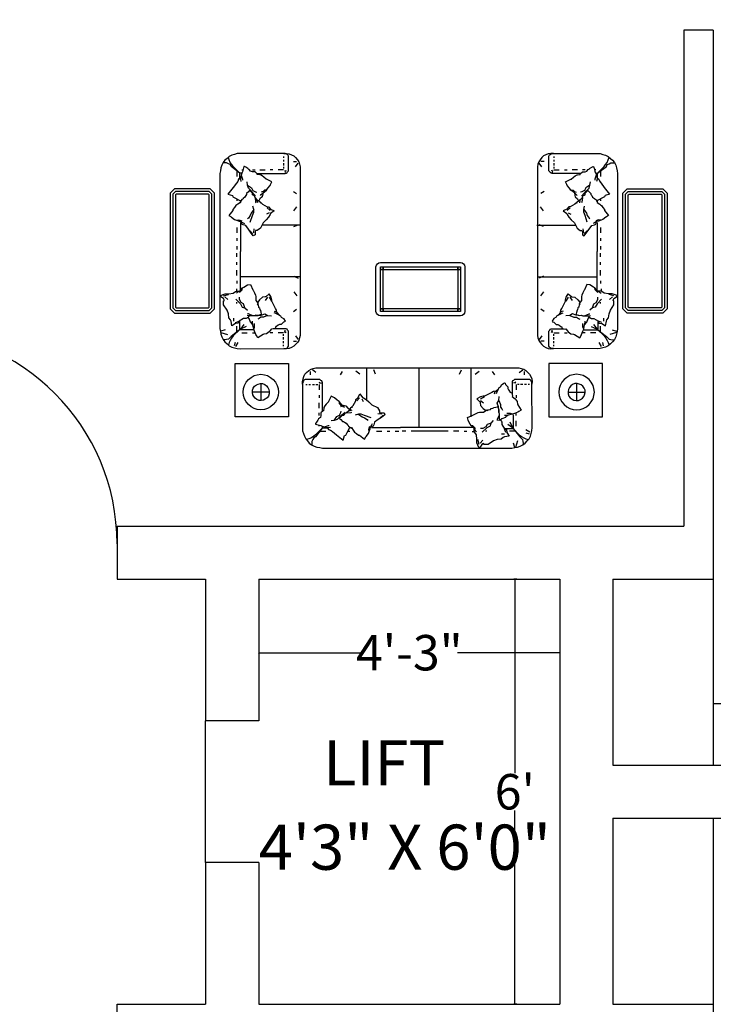
# Model space of a CAD drawing. Units: inches. Extents: x -113 to 5399, y -1393 to 3302.
# Tile 16 of 40: x 1779 to 1896, y 426 to 592. Entities that reach past the tile are written whole.
import ezdxf

# ---------------------------------------------------------------- set-up
doc = ezdxf.new("R2010")
doc.units = ezdxf.units.IN
doc.header["$MEASUREMENT"] = 0
doc.layers.add('24', color=7, linetype='Continuous')
for name, color, linetype, lineweight in [('A-ANNO-DIMS', 254, 'Continuous', 18), ('A-AREA-IDEN', 4, 'Continuous', 18), ('doors', 2, 'Continuous', 25), ('furniture', 131, 'Continuous', 18), ('walls', 1, 'Continuous', 25)]:
    doc.layers.add(name, color=color, linetype=linetype, lineweight=lineweight)
doc.styles.get("Standard").update_dxf_attribs({"font": 'arial.ttf'})
doc.dimstyles.get("Standard").update_dxf_attribs({"dimtxt": 6, "dimasz": 0.18, "dimexe": 0.18, "dimexo": 0.0625, "dimgap": 0.09, "dimtad": 0, "dimtih": 1, "dimtoh": 1, "dimdec": 1, "dimzin": 0, "dimdsep": 46, "dimlunit": 4, "dimtxsty": 'Standard', "dimblk": 'ARCHTICK', "dimcen": 0.09, "dimadec": 0, "dimazin": 0, "dimtfac": 1, "dimtdec": 1, "dimtofl": 0, "dimtmove": 0, "dimatfit": 3, "dimfxl": 1, "dimtolj": 1, "dimtzin": 0, "dimarcsym": 0})

# ---------------------------------------------------------------- blocks, each defined once
blk = doc.blocks.new('*U3')
for p, q in [((0, 0), (0, -6)), ((36, 0), (36, -6))]:
    blk.add_line(p, q)
blk.add_lwpolyline([(0, 0), (0, 36), (1.75, 36), (1.75, 0)], close=True)
blk.add_arc((0, 0), 36, 0, 90)
blk = doc.blocks.new('DL13712')
at = {"layer": '24'}
for p, q in [((33, 28.5), (-34, 28.5)), ((33.5, -29.5), (-10, -29.5))]:
    blk.add_line(p, q, dxfattribs=at)
blk = doc.blocks.new('DL13976')
at = {"layer": '24'}
for p, q in [((-16, 11), (-13.5, 14)), ((-13.5, 14), (-10.5, 16.5)), ((-10.5, 16.5), (-7, 18.5)), ((-7, 18.5), (-3.5, 19.5)), ((-3.5, 19.5), (0.5, 20)), ((0.5, 20), (4.5, 19.5)), ((4.5, 19.5), (8, 18.5)), ((8, 18.5), (11.5, 16.5)), ((11.5, 16.5), (14.5, 14)), ((14.5, 14), (17, 11)), ((-19.5, 0), (-19, 4)), ((-19, -4), (-19.5, 0)), ((-19, 4), (-18, 7.5)), ((-18, 7.5), (-16, 11)), ((-9, 2), (-8, 4.5)), ((-9, -0.5), (-9, 2)), ((-9, 0), (10, 0)), ((-8, 4.5), (-6.5, 6.5)), ((-6.5, 6.5), (-4.5, 8)), ((-5.5, 0), (6.5, 0)), ((-4.5, 8), (-2.5, 9)), ((-2.5, 9), (0, 9.5)), ((0, 9.5), (2.5, 9.5)), ((0.5, -9.5), (0.5, 9.5)), ((0.5, -6), (0.5, 6)), ((2.5, 9.5), (5, 8.5)), ((5, 8.5), (7, 7)), ((7, 7), (8.5, 5)), ((8.5, 5), (9.5, 3)), ((9.5, 3), (10, 0.5)), ((10, 0.5), (10, -2)), ((17, 11), (19, 7.5)), ((19, 7.5), (20, 4)), ((20, 4), (20.5, 0)), ((20.5, 0), (20, -4)), ((-18, -7.5), (-19, -4)), ((-16, -11), (-18, -7.5)), ((-13.5, -14), (-16, -11)), ((-8.5, -3), (-9, -0.5)), ((-7.5, -5), (-8.5, -3)), ((-6, -7), (-7.5, -5)), ((-4, -8.5), (-6, -7)), ((-1.5, -9.5), (-4, -8.5)), ((1, -9.5), (-1.5, -9.5)), ((3.5, -9), (1, -9.5)), ((5.5, -8), (3.5, -9)), ((7.5, -6.5), (5.5, -8)), ((9, -4.5), (7.5, -6.5)), ((10, -2), (9, -4.5)), ((17, -11), (14.5, -14)), ((19, -7.5), (17, -11)), ((20, -4), (19, -7.5)), ((-10.5, -16.5), (-13.5, -14)), ((-7, -18.5), (-10.5, -16.5)), ((-3.5, -19.5), (-7, -18.5)), ((0.5, -20), (-3.5, -19.5)), ((4.5, -19.5), (0.5, -20)), ((8, -18.5), (4.5, -19.5)), ((11.5, -16.5), (8, -18.5)), ((14.5, -14), (11.5, -16.5))]:
    blk.add_line(p, q, dxfattribs=at)
blk = doc.blocks.new('DL13329')
at = {"layer": '24'}
for p, q in [((0, 0), (0, -60)), ((60, 0), (0, 0)), ((60, -60), (60, 0)), ((0, -60), (60, -60))]:
    blk.add_line(p, q, dxfattribs=at)
blk = doc.blocks.new('DL13303')
at = {"layer": '24'}
for p, q in [((-70, 20), (-65, 25)), ((-65, 25), (65, 25)), ((65, 25), (70, 20)), ((-70, -20), (-70, 20)), ((-67, 19), (-64, 22)), ((-67, -19), (-67, 19)), ((-64, 22), (64, 22)), ((-64, 18), (-63, 19)), ((-64, -18), (-64, 18)), ((-63, 19), (63, 19)), ((63, 19), (64, 18)), ((64, 22), (67, 19)), ((64, 18), (64, -18)), ((67, 19), (67, -19)), ((70, 20), (70, -20)), ((-65, -25), (-70, -20)), ((-64, -22), (-67, -19)), ((-63, -19), (-64, -18)), ((64, -22), (-64, -22)), ((63, -19), (-63, -19)), ((64, -18), (63, -19)), ((67, -19), (64, -22)), ((70, -20), (65, -25)), ((65, -25), (-65, -25))]:
    blk.add_line(p, q, dxfattribs=at)
blk = doc.blocks.new('DL12701')
at = {"layer": '24'}
for p, q in [((-96.5, 43.5), (-93.5, 44.5)), ((-93.5, 44.5), (-90, 45)), ((-90, 45), (-87, 45.5)), ((-87, 45.5), (0, 45.5)), ((0, 45.5), (87, 45.5)), ((50, 45), (48, 39.5)), ((51.5, 44.5), (50, 45)), ((53.5, 41.5), (51.5, 44.5)), ((87, 45.5), (90.5, 45)), ((88.5, 39.5), (90, 44.5)), ((90.5, 45), (93.5, 44.5)), ((91.5, 44.5), (94, 37)), ((93.5, 44.5), (96.5, 43.5)), ((-107.5, 32), (-106, 35)), ((-106, 35), (-104, 37.5)), ((-102.5, 35), (-105, 36)), ((-104, 37.5), (-102, 40)), ((-99.5, 34), (-102.5, 35)), ((-102, 40), (-99.5, 42)), ((-99.5, 42), (-96.5, 43.5)), ((-97, 32), (-99.5, 34)), ((-99, 40), (-99, 42)), ((-99, 38), (-99, 40)), ((-98, 36), (-99, 38)), ((-97, 34), (-98, 36)), ((-95, 33), (-97, 34)), ((-69.5, 32), (-67.5, 33.5)), ((-67.5, 33.5), (-64, 36.5)), ((-64, 36.5), (-62.5, 31.5)), ((-45.5, 31), (-40, 35.5)), ((-40, 35.5), (-38.5, 33)), ((48, 35.5), (47.5, 30.5)), ((48, 39.5), (48, 35.5)), ((50.5, 41.5), (49, 36)), ((51.5, 40), (54.5, 36.5)), ((55.5, 40.5), (53.5, 41.5)), ((56, 41.5), (55.5, 40.5)), ((60.5, 41.5), (56, 41.5)), ((66.5, 37.5), (60.5, 41.5)), ((70.5, 36), (66.5, 37.5)), ((75, 35.5), (70.5, 36)), ((77.5, 33.5), (75, 35.5)), ((79, 33), (77.5, 33.5)), ((96, 33), (97.5, 34.5)), ((96.5, 43.5), (99.5, 42)), ((97.5, 34.5), (99, 36)), ((98, 32.5), (100.5, 34)), ((99, 36), (99.5, 38)), ((99.5, 42), (102, 40)), ((100, 40), (99.5, 42)), ((99.5, 38), (100, 40)), ((100.5, 34), (103, 35)), ((102, 40), (104.5, 37.5)), ((103, 35), (106, 36)), ((104.5, 37.5), (106.5, 35)), ((106.5, 35), (108, 32)), ((-109.5, 26), (-108.5, 29)), ((-109.5, 22.5), (-109.5, 26)), ((-109.5, -26.5), (-109.5, 22.5)), ((-108.5, 29), (-107.5, 32)), ((-95, 30.5), (-97, 32)), ((-87.5, 23), (-95, 33)), ((-87.5, 23), (-95, 30.5)), ((-89.5, 26.5), (-83.5, 26.5)), ((-87.5, 21), (-87.5, 23)), ((-81.5, 23), (-87.5, 23)), ((-85, 21.5), (-82, 22.5)), ((-82, 22.5), (-80.5, 24.5)), ((-82, 22.5), (-80.5, 22.5)), ((-80.5, 24.5), (-78, 25.5)), ((-80.5, 24.5), (-80.5, 23.5)), ((-80.5, 22.5), (-78, 22)), ((-78, 25.5), (-76, 27)), ((-77, 25.5), (-77, 25.5)), ((-76, 27), (-71.5, 30.5)), ((-71.5, 30.5), (-69.5, 32)), ((-62.5, 31.5), (-61, 31)), ((-61, 31), (-59.5, 28)), ((-59.5, 28), (-57.5, 24.5)), ((-58, 26.5), (-56.5, 26.5)), ((-58, 21), (-54.5, 23)), ((-57.5, 24.5), (-56.5, 22)), ((-56.5, 22.5), (-54.5, 22.5)), ((-54.5, 22.5), (-52.5, 25.5)), ((-54.5, 23), (-54.5, 22.5)), ((-54, 22.5), (-54, 22.5)), ((-52.5, 25.5), (-52, 26.5)), ((-52, 26.5), (-51, 27.5)), ((-51, 27.5), (-49, 29)), ((-49, 29), (-46.5, 31)), ((-46.5, 31), (-45.5, 31)), ((-38.5, 33), (-38, 32.5)), ((-38, 32.5), (-35.5, 29)), ((-35.5, 29), (-34.5, 27)), ((-34.5, 27), (-35, 24.5)), ((-35, 24.5), (-34.5, 23)), ((-34.5, 27), (-33.5, 24)), ((-34.5, 23), (-34, 21)), ((-33.5, 24), (-33, 22)), ((-32, 22.5), (0.5, 22.5)), ((-26.5, 26.5), (-20.5, 26.5)), ((-14.5, 26.5), (-11.5, 26.5)), ((-5.5, 26.5), (-1.5, 26.5)), ((44, 22.5), (0.5, 22.5)), ((6.5, 26.5), (2.5, 26.5)), ((15.5, 26.5), (12.5, 26.5)), ((27.5, 26.5), (21.5, 26.5)), ((33.5, 26.5), (36.5, 26.5)), ((42.5, 27), (45, 27)), ((45, 23.5), (43.5, 22)), ((45.5, 28), (45, 27)), ((45, 27), (45, 23.5)), ((45, 23.5), (46.5, 26)), ((46.5, 23.5), (45, 22)), ((47.5, 30.5), (45.5, 28)), ((46.5, 26), (47.5, 27)), ((54.5, 23.5), (52, 23.5)), ((54, 27.5), (59.5, 22.5)), ((58, 21.5), (54.5, 23.5)), ((59, 26.5), (57.5, 26.5)), ((59.5, 22.5), (63, 20.5)), ((79, 30), (75.5, 30)), ((76, 19), (79, 24)), ((84, 32), (79, 33)), ((80.5, 28), (79, 24)), ((79, 24), (81, 24.5)), ((79, 23.5), (88.5, 23.5)), ((81, 24.5), (81.5, 28)), ((81.5, 28), (84, 32)), ((82.5, 18.5), (88, 22.5)), ((90.5, 26.5), (84.5, 26.5)), ((85, 16), (88, 22.5)), ((88.5, 23.5), (96, 33)), ((88.5, 23.5), (95.5, 30.5)), ((88.5, 8), (88.5, 23.5)), ((95.5, 30.5), (98, 32.5)), ((103, 28.5), (106.5, 29.5)), ((107.5, 27.5), (103, 25)), ((108, 32), (109, 29)), ((109, 29), (109.5, 26)), ((109.5, 26), (110, 22.5)), ((110, 22.5), (109.5, -26.5)), ((-95, 18.5), (-92, 19.5)), ((-95, 18), (-95, 18.5)), ((-94, 16.5), (-95, 18)), ((-92.5, 14), (-94, 16.5)), ((-92, 13.5), (-92.5, 14)), ((-92, 19.5), (-89, 20)), ((-91.5, 12.5), (-92, 13.5)), ((-89.5, 11), (-91.5, 12.5)), ((-91, 21), (-91, 19.5)), ((-89, 20), (-87.5, 21)), ((-87.5, 21), (-85, 21.5)), ((-85, 21.5), (-80.5, 20)), ((-80.5, 20), (-79.5, 20)), ((-74, 14.5), (-77.5, 15)), ((-70.5, 13.5), (-74, 14.5)), ((-74, 14.5), (-71, 10)), ((-67.5, 10.5), (-70.5, 13.5)), ((-68, 12), (-67.5, 12.5)), ((-65, 9), (-68, 12)), ((-67.5, 12.5), (-66.5, 13.5)), ((-66.5, 13.5), (-64.5, 15.5)), ((-64.5, 15.5), (-63.5, 15.5)), ((-63.5, 15.5), (-62.5, 16.5)), ((-62.5, 16.5), (-60.5, 17.5)), ((-60.5, 17.5), (-59, 19.5)), ((-59, 19.5), (-58.5, 19.5)), ((-58.5, 19.5), (-58, 21)), ((-42.5, 10.5), (-40, 11.5)), ((-40, 11.5), (-37, 13.5)), ((-32.5, 11.5), (-40, 9)), ((-37, 13.5), (-36, 14.5)), ((-30, 21), (-33, 22)), ((-33, 22), (-31.5, 19.5)), ((-31.5, 19.5), (-31, 18)), ((-29.5, 19.5), (-30, 21)), ((-28.5, 16.5), (-29.5, 19.5)), ((-24.5, 13.5), (-28.5, 16.5)), ((-21, 11), (-24.5, 13.5)), ((-19, 8.5), (-22.5, 11.5)), ((38, 14), (37.5, 11)), ((40.5, 18.5), (38, 14.5)), ((38, 14.5), (38, 14)), ((41.5, 20), (40.5, 18.5)), ((43.5, 22), (41.5, 20)), ((43.5, 20.5), (41.5, 20)), ((45, 22), (43.5, 20.5)), ((59.5, 19), (58, 21.5)), ((64, 17.5), (59.5, 19)), ((63, 20.5), (64, 17.5)), ((64, 17.5), (66.5, 14.5)), ((70.5, 13.5), (70.5, 14.5)), ((73, 8.5), (70.5, 13.5)), ((73, 13), (72.5, 15)), ((73, 12.5), (75, 14.5)), ((73, 12.5), (73, 13)), ((73, 8.5), (73, 12.5)), ((76, 12.5), (74, 14)), ((75, 14.5), (76, 16)), ((75.5, 16), (76, 16.5)), ((76, 16), (76, 19)), ((80, 11), (76, 12.5)), ((92, 21), (92, 15)), ((-91, 9), (-91, 6)), ((-91, 0.5), (-91, -5.5)), ((-89, 9), (-89.5, 11)), ((-89, 8.5), (-89, 9)), ((-89, 6), (-89, 8.5)), ((-86.5, 3.5), (-89, 6)), ((-87, 3.5), (-87, -26.5)), ((-86, 3.5), (-86.5, 3.5)), ((-85.5, 0.5), (-86, 3.5)), ((-85.5, 0), (-85.5, 0.5)), ((-84.5, -2), (-85.5, 0)), ((-71, 10), (-68, 8.5)), ((-68, 8.5), (-66.5, 5.5)), ((-61.5, 5.5), (-67.5, 10.5)), ((-66.5, 5.5), (-66, 4)), ((-63, 9), (-65, 9)), ((-62.5, 0), (-63.5, -1)), ((-62, 6.5), (-63, 9)), ((-60, 6), (-62, 6.5)), ((-61, -2), (-58.5, 0.5)), ((-57.5, 3.5), (-60, 6)), ((-60, 6), (-55, 5.5)), ((-58.5, 0.5), (-55.5, 2)), ((-56.5, 3.5), (-57.5, 3.5)), ((-57.5, 3.5), (-56, 1.5)), ((-54, 3), (-56.5, 3.5)), ((-56, 1.5), (-55, 0)), ((-55, 5.5), (-54, 5)), ((-55, 0), (-52.5, -2.5)), ((-46.5, 7.5), (-50.5, 8.5)), ((-46.5, 7.5), (-42.5, 10.5)), ((-43.5, 7.5), (-46.5, 7.5)), ((-40, 9), (-43.5, 7.5)), ((-31.5, -3), (-25.5, 0)), ((-25.5, 0), (-23, 3.5)), ((-20.5, 7.5), (-25, 7)), ((-23, 5.5), (-21.5, 6)), ((-23, 3.5), (-23, 5.5)), ((-21.5, 6), (-18, 6)), ((-17, 8), (-21, 11)), ((-18, 6), (-17, 8)), ((37.5, 11), (43.5, 8.5)), ((43.5, 8.5), (44, 8)), ((44, 8), (47, 6.5)), ((47, 6.5), (49.5, 5.5)), ((49.5, 5.5), (51, 5)), ((51, 5), (52.5, 5)), ((52, -2.5), (55, 1)), ((52.5, 5), (55.5, 5)), ((55, 1), (57.5, 3)), ((55.5, 5), (55.5, 5)), ((55.5, 5), (59, 2.5)), ((59, 2.5), (60, 3.5)), ((60, 3.5), (60, 2.5)), ((60, 2.5), (63, 2)), ((63, 2), (64, 1)), ((64, 1), (66, 0.5)), ((66, 0.5), (66.5, 0)), ((66.5, 0), (69, -0.5)), ((71.5, -1), (72.5, 2.5)), ((72, 5), (73, 6.5)), ((73, 5.5), (72, -1)), ((72.5, 2.5), (72, 5)), ((73, 6.5), (73, 8.5)), ((74.5, -0.5), (76, 1.5)), ((76, 1.5), (76.5, 3)), ((80.5, 9), (79, 9)), ((80.5, 10.5), (80, 11)), ((83, 8.5), (80.5, 10.5)), ((83, 8.5), (80.5, 9)), ((84, 6.5), (81.5, 6.5)), ((85, 8), (83, 8.5)), ((85.5, 6.5), (84, 6.5)), ((88, 7.5), (85, 8)), ((88, 7.5), (85.5, 6.5)), ((90, 6.5), (88, 7.5)), ((94, 5), (90, 6.5)), ((92, 9), (92, 6)), ((95, 4.5), (94, 5)), ((94, -3), (97.5, 3)), ((97.5, 3), (95, 4.5)), ((-91, -14), (-91, -11)), ((-83, -4), (-84.5, -2)), ((-80.5, -6.5), (-83, -4)), ((-80.5, -7), (-80.5, -6.5)), ((-77.5, -13), (-80.5, -7)), ((-73.5, -11), (-74.5, -11.5)), ((-70.5, -8.5), (-73.5, -11)), ((-68.5, -7), (-70.5, -8.5)), ((-68.5, -4.5), (-67, -3)), ((-66.5, -4.5), (-68.5, -7)), ((-68.5, -7), (-68.5, -4.5)), ((-67, -3), (-66, -1)), ((-65.5, -3), (-66.5, -4.5)), ((-63.5, -1), (-65.5, -3)), ((-65.5, -3), (-62.5, -2.5)), ((-62.5, -2.5), (-61, -2)), ((-54, -0.5), (-53.5, -0.5)), ((-52.5, -2.5), (-49.5, -7.5)), ((-49.5, -7.5), (-49.5, -9)), ((-49.5, -9), (-47, -11.5)), ((-45.5, -11), (-48.5, -7.5)), ((-43, -10), (-41.5, -7)), ((-42, -11.5), (-41, -11)), ((-41, -11), (-38, -9)), ((-38, -9), (-35, -6.5)), ((-35, -6.5), (-31.5, -3)), ((48, -10), (51.5, -6)), ((52, -12), (48, -10)), ((51.5, -5.5), (52, -2.5)), ((51.5, -6), (51.5, -5.5)), ((52, -8), (55.5, -5.5)), ((52, -10), (56.5, -12.5)), ((69, -0.5), (70.5, -1)), ((70.5, -1), (71.5, -1)), ((72, -1), (70.5, -5)), ((70.5, -5), (72.5, -8)), ((72.5, -8), (74.5, -3.5)), ((72.5, -8), (73, -12.5)), ((74.5, -3.5), (74.5, -0.5)), ((87.5, -12.5), (89.5, -11)), ((89.5, -11), (91, -10)), ((91, -10), (92, -8.5)), ((92, -8.5), (93, -7)), ((92, -14), (92, -11)), ((93, -7), (93.5, -4)), ((93.5, -4), (94, -3)), ((-91, -26), (-91, -20)), ((-74.5, -11.5), (-77.5, -13)), ((-47, -11.5), (-45, -15.5)), ((-45, -15.5), (-42, -11.5)), ((55, -13), (52, -12)), ((56.5, -13), (55, -13)), ((62.5, -16), (56.5, -13)), ((64.5, -17), (62.5, -16)), ((64, -16.5), (64, -16.5)), ((66.5, -18), (64.5, -17)), ((69, -18.5), (66.5, -18)), ((67.5, -15.5), (68.5, -18)), ((68.5, -18), (69, -18.5)), ((69, -18.5), (72, -21)), ((70, -16.5), (69.5, -15.5)), ((72, -21), (70, -16.5)), ((72, -21), (73, -22.5)), ((82.5, -21.5), (83.5, -20)), ((82.5, -22.5), (82.5, -21.5)), ((83.5, -20), (85, -18)), ((85, -17.5), (87, -16.5)), ((85, -18), (85, -17.5)), ((87, -16.5), (88, -13)), ((88, -13), (87.5, -12.5)), ((87.5, -26.5), (87.5, -14.5)), ((92, -26), (92, -20)), ((-109.5, -28), (-109.5, -26.5)), ((-109.5, -26.5), (-109.5, -29.5)), ((-109, -29), (-109.5, -28)), ((-109.5, -29.5), (-109, -32.5)), ((-108.5, -30), (-109, -29)), ((-109, -32.5), (-108, -35)), ((-108, -31), (-108.5, -30)), ((-106.5, -31.5), (-108, -31)), ((-105.5, -31.5), (-106.5, -31.5)), ((-106, -26), (-104.5, -26)), ((-104.5, -31.5), (-105.5, -31.5)), ((-92, -31.5), (-104.5, -31.5)), ((-102.5, -26), (-100.5, -26)), ((-98.5, -26), (-96, -26)), ((-94.5, -26), (-92.5, -26)), ((-91, -31.5), (-92, -31.5)), ((-90, -31.5), (-91, -31.5)), ((-90.5, -27.5), (-88, -28)), ((-90.5, -28), (-90, -29)), ((-89, -30.5), (-90, -31.5)), ((-88, -30), (-89, -30.5)), ((-87.5, -29), (-88, -30)), ((-87, -28), (-87.5, -29)), ((-87, -26.5), (-87, -28)), ((73, -22.5), (74.5, -23.5)), ((74.5, -23.5), (76, -26)), ((76, -26), (79, -28)), ((79, -28), (79.5, -27.5)), ((79.5, -27.5), (80, -26)), ((80, -26), (82.5, -23.5)), ((82.5, -23.5), (82.5, -22.5)), ((87.5, -28), (87.5, -26.5)), ((87.5, -29), (87.5, -28)), ((88, -30), (87.5, -29)), ((89, -30.5), (88, -30)), ((91.5, -27.5), (89, -28)), ((90, -31.5), (89, -30.5)), ((91, -31.5), (90, -31.5)), ((91.5, -28), (91, -29)), ((92.5, -31.5), (91, -31.5)), ((104.5, -31.5), (92.5, -31.5)), ((95.5, -26), (93.5, -26)), ((99.5, -26), (97, -26)), ((103.5, -26), (101.5, -26)), ((106, -31.5), (104.5, -31.5)), ((107, -26), (105.5, -26)), ((107, -31.5), (106, -31.5)), ((108, -31), (107, -31.5)), ((109, -30), (108, -31)), ((108.5, -35), (109.5, -32.5)), ((109.5, -29), (109, -30)), ((110, -29.5), (109.5, -26.5)), ((109.5, -26.5), (109.5, -28)), ((109.5, -28), (109.5, -29)), ((109.5, -32.5), (110, -29.5)), ((-108, -35), (-107, -37.5)), ((-107, -37.5), (-105, -39.5)), ((-105, -39.5), (-102.5, -41.5)), ((-102.5, -41.5), (-100, -43)), ((-100.5, -37), (-100.5, -40.5)), ((-100, -43), (-97.5, -44)), ((-94.5, -39.5), (-98.5, -42.5)), ((-97.5, -44), (-94.5, -44.5)), ((-67, -37), (-64.5, -40.5)), ((-45, -37.5), (-49.5, -41)), ((-27.5, -37.5), (-29.5, -42.5)), ((28.5, -37.5), (30.5, -42.5)), ((46, -37.5), (50.5, -41)), ((68, -37), (65.5, -40.5)), ((95, -44.5), (97.5, -44)), ((95.5, -39.5), (99.5, -42.5)), ((97.5, -44), (100.5, -43)), ((100.5, -43), (103, -41.5)), ((101.5, -37), (101.5, -40.5)), ((103, -41.5), (105, -39.5)), ((105, -39.5), (107, -37.5)), ((107, -37.5), (108.5, -35)), ((-94.5, -44.5), (0, -44.5)), ((0, -44.5), (95, -44.5))]:
    blk.add_line(p, q, dxfattribs=at)
blk = doc.blocks.new('DL13707')
at = {"layer": '24'}
for p, q in [((0, -33.5), (0, 33.5)), ((-58.5, -33.5), (-58.5, 21.5)), ((58.5, -33.5), (58.5, 2))]:
    blk.add_line(p, q, dxfattribs=at)
blk = doc.blocks.new('DL13651')
at = {"layer": '24'}
for p, q in [((-50.5, 25), (-50, 27)), ((-50.5, -25), (-50.5, 25)), ((-50, 27), (-49, 28.5)), ((-49, 28.5), (-47.5, 29.5)), ((-47.5, 29.5), (-45.5, 30)), ((-45.5, 30), (44.5, 30)), ((-45.5, 24.5), (-45.5, 25)), ((-45.5, 25), (-45, 25)), ((-45.5, -24.5), (-45.5, 24.5)), ((-45, 25), (44, 25)), ((-42.5, -24.5), (-42.5, 24.5)), ((-42.5, 24.5), (-42.5, 22)), ((41.5, 22), (41.5, 24.5)), ((41.5, 24.5), (41.5, -24.5)), ((44, 25), (44.5, 25)), ((44.5, 30), (46.5, 29.5)), ((44.5, 25), (44.5, 24.5)), ((44.5, 24.5), (44.5, -24.5)), ((46.5, 29.5), (48, 28.5)), ((48, 28.5), (49, 27)), ((49, 27), (49.5, 25)), ((49.5, 25), (49.5, -25)), ((-45, 22), (44, 22)), ((-42.5, 22), (-45, 22)), ((44, 22), (41.5, 22)), ((44, -22), (-45, -22)), ((-45, -22), (-42.5, -22)), ((-42.5, -22), (-42.5, -24.5)), ((41.5, -24.5), (41.5, -22)), ((41.5, -22), (44, -22)), ((-50, -27), (-50.5, -25)), ((-49, -28.5), (-50, -27)), ((-47.5, -29.5), (-49, -28.5)), ((-45.5, -30), (-47.5, -29.5)), ((-45.5, -25), (-45.5, -24.5)), ((-45, -25), (-45.5, -25)), ((44.5, -30), (-45.5, -30)), ((44, -25), (-45, -25)), ((44.5, -25), (44, -25)), ((44.5, -24.5), (44.5, -25)), ((46.5, -29.5), (44.5, -30)), ((48, -28.5), (46.5, -29.5)), ((49, -27), (48, -28.5)), ((49.5, -25), (49, -27))]:
    blk.add_line(p, q, dxfattribs=at)
blk = doc.blocks.new('DL12263')
at = {"layer": '24'}
for p, q in [((-115.5, 43.5), (-112.5, 44.5)), ((-112.5, 44.5), (-109, 45)), ((-109, 45), (-106, 45.5)), ((-106, 45.5), (-19, 45.5)), ((-19, 45.5), (106.5, 45.5)), ((69.5, 45), (67.5, 39.5)), ((71, 44.5), (69.5, 45)), ((73, 41.5), (71, 44.5)), ((106.5, 45.5), (110, 45)), ((108, 39.5), (109.5, 44.5)), ((110, 45), (113, 44.5)), ((111, 44.5), (113.5, 37)), ((113, 44.5), (116, 43.5)), ((-126.5, 32), (-125, 35)), ((-125, 35), (-123, 37.5)), ((-121.5, 35), (-124, 36)), ((-123, 37.5), (-121, 40)), ((-118.5, 34), (-121.5, 35)), ((-121, 40), (-118.5, 42)), ((-118.5, 42), (-115.5, 43.5)), ((-116, 32), (-118.5, 34)), ((-118, 40), (-118, 42)), ((-118, 38), (-118, 40)), ((-117, 36), (-118, 38)), ((-116, 34), (-117, 36)), ((-114, 33), (-116, 34)), ((-88.5, 32), (-86.5, 33.5)), ((-86.5, 33.5), (-83, 36.5)), ((-83, 36.5), (-81.5, 31.5)), ((-64.5, 31), (-59, 35.5)), ((-59, 35.5), (-57.5, 33)), ((67.5, 35.5), (67, 30.5)), ((67.5, 39.5), (67.5, 35.5)), ((70, 41.5), (68.5, 36)), ((71, 40), (74, 36.5)), ((75, 40.5), (73, 41.5)), ((75.5, 41.5), (75, 40.5)), ((80, 41.5), (75.5, 41.5)), ((86, 37.5), (80, 41.5)), ((90, 36), (86, 37.5)), ((94.5, 35.5), (90, 36)), ((97, 33.5), (94.5, 35.5)), ((98.5, 33), (97, 33.5)), ((115.5, 33), (117, 34.5)), ((116, 43.5), (119, 42)), ((117, 34.5), (118.5, 36)), ((117.5, 32.5), (120, 34)), ((118.5, 36), (119, 38)), ((119, 42), (121.5, 40)), ((119.5, 40), (119, 42)), ((119, 38), (119.5, 40)), ((120, 34), (122.5, 35)), ((121.5, 40), (124, 37.5)), ((122.5, 35), (125.5, 36)), ((124, 37.5), (126, 35)), ((126, 35), (127.5, 32)), ((-128.5, 26), (-127.5, 29)), ((-128.5, 22.5), (-128.5, 26)), ((-128.5, -26.5), (-128.5, 22.5)), ((-127.5, 29), (-126.5, 32)), ((-114, 30.5), (-116, 32)), ((-106.5, 23), (-114, 33)), ((-106.5, 23), (-114, 30.5)), ((-108.5, 26.5), (-102.5, 26.5)), ((-106.5, 21), (-106.5, 23)), ((-100.5, 23), (-106.5, 23)), ((-104, 21.5), (-101, 22.5)), ((-101, 22.5), (-99.5, 24.5)), ((-101, 22.5), (-99.5, 22.5)), ((-99.5, 24.5), (-97, 25.5)), ((-99.5, 24.5), (-99.5, 23.5)), ((-99.5, 22.5), (-97, 22)), ((-97, 25.5), (-95, 27)), ((-96, 25.5), (-96, 25.5)), ((-95, 27), (-90.5, 30.5)), ((-90.5, 30.5), (-88.5, 32)), ((-81.5, 31.5), (-80, 31)), ((-80, 31), (-78.5, 28)), ((-78.5, 28), (-76.5, 24.5)), ((-77, 26.5), (-75.5, 26.5)), ((-77, 21), (-73.5, 23)), ((-76.5, 24.5), (-75.5, 22)), ((-75.5, 22.5), (-73.5, 22.5)), ((-73.5, 22.5), (-71.5, 25.5)), ((-73.5, 23), (-73.5, 22.5)), ((-73, 22.5), (-73, 22.5)), ((-71.5, 25.5), (-71, 26.5)), ((-71, 26.5), (-70, 27.5)), ((-70, 27.5), (-68, 29)), ((-68, 29), (-65.5, 31)), ((-65.5, 31), (-64.5, 31)), ((-57.5, 33), (-57, 32.5)), ((-57, 32.5), (-54.5, 29)), ((-54.5, 29), (-53.5, 27)), ((-53.5, 27), (-54, 24.5)), ((-54, 24.5), (-53.5, 23)), ((-53.5, 27), (-52.5, 24)), ((-53.5, 23), (-53, 21)), ((-52.5, 24), (-52, 22)), ((-51, 22.5), (-18.5, 22.5)), ((-45.5, 26.5), (-39.5, 26.5)), ((-33.5, 26.5), (-30.5, 26.5)), ((-24.5, 26.5), (-20.5, 26.5)), ((63.5, 22.5), (-18.5, 22.5)), ((-12.5, 26.5), (-16.5, 26.5)), ((35, 26.5), (-6.5, 26.5)), ((47, 26.5), (41, 26.5)), ((53, 26.5), (56, 26.5)), ((62, 27), (64.5, 27)), ((64.5, 23.5), (63, 22)), ((65, 28), (64.5, 27)), ((64.5, 27), (64.5, 23.5)), ((64.5, 23.5), (66, 26)), ((66, 23.5), (64.5, 22)), ((67, 30.5), (65, 28)), ((66, 26), (67, 27)), ((74, 23.5), (71.5, 23.5)), ((73.5, 27.5), (79, 22.5)), ((77.5, 21.5), (74, 23.5)), ((78.5, 26.5), (77, 26.5)), ((79, 22.5), (82.5, 20.5)), ((98.5, 30), (95, 30)), ((95.5, 19), (98.5, 24)), ((103.5, 32), (98.5, 33)), ((100, 28), (98.5, 24)), ((98.5, 24), (100.5, 24.5)), ((98.5, 23.5), (108, 23.5)), ((100.5, 24.5), (101, 28)), ((101, 28), (103.5, 32)), ((102, 18.5), (107.5, 22.5)), ((110, 26.5), (104, 26.5)), ((104.5, 16), (107.5, 22.5)), ((108, 23.5), (115.5, 33)), ((108, 23.5), (115, 30.5)), ((108, 8), (108, 23.5)), ((115, 30.5), (117.5, 32.5)), ((122.5, 28.5), (126, 29.5)), ((127, 27.5), (122.5, 25)), ((127.5, 32), (128.5, 29)), ((128.5, 29), (129, 26)), ((129, 26), (129.5, 22.5)), ((129.5, 22.5), (129, -26.5)), ((-114, 18.5), (-111, 19.5)), ((-114, 18), (-114, 18.5)), ((-113, 16.5), (-114, 18)), ((-111.5, 14), (-113, 16.5)), ((-111, 13.5), (-111.5, 14)), ((-111, 19.5), (-108, 20)), ((-110.5, 12.5), (-111, 13.5)), ((-108.5, 11), (-110.5, 12.5)), ((-110, 21), (-110, 19.5)), ((-108, 20), (-106.5, 21)), ((-106.5, 21), (-104, 21.5)), ((-104, 21.5), (-99.5, 20)), ((-99.5, 20), (-98.5, 20)), ((-93, 14.5), (-96.5, 15)), ((-89.5, 13.5), (-93, 14.5)), ((-93, 14.5), (-90, 10)), ((-86.5, 10.5), (-89.5, 13.5)), ((-87, 12), (-86.5, 12.5)), ((-84, 9), (-87, 12)), ((-86.5, 12.5), (-85.5, 13.5)), ((-85.5, 13.5), (-83.5, 15.5)), ((-83.5, 15.5), (-82.5, 15.5)), ((-82.5, 15.5), (-81.5, 16.5)), ((-81.5, 16.5), (-79.5, 17.5)), ((-79.5, 17.5), (-78, 19.5)), ((-78, 19.5), (-77.5, 19.5)), ((-77.5, 19.5), (-77, 21)), ((-61.5, 10.5), (-59, 11.5)), ((-59, 11.5), (-56, 13.5)), ((-51.5, 11.5), (-59, 9)), ((-56, 13.5), (-55, 14.5)), ((-49, 21), (-52, 22)), ((-52, 22), (-50.5, 19.5)), ((-50.5, 19.5), (-50, 18)), ((-48.5, 19.5), (-49, 21)), ((-47.5, 16.5), (-48.5, 19.5)), ((-43.5, 13.5), (-47.5, 16.5)), ((-40, 11), (-43.5, 13.5)), ((-38, 8.5), (-41.5, 11.5)), ((57.5, 14), (57, 11)), ((60, 18.5), (57.5, 14.5)), ((57.5, 14.5), (57.5, 14)), ((61, 20), (60, 18.5)), ((63, 22), (61, 20)), ((63, 20.5), (61, 20)), ((64.5, 22), (63, 20.5)), ((79, 19), (77.5, 21.5)), ((83.5, 17.5), (79, 19)), ((82.5, 20.5), (83.5, 17.5)), ((83.5, 17.5), (86, 14.5)), ((90, 13.5), (90, 14.5)), ((92.5, 8.5), (90, 13.5)), ((92.5, 13), (92, 15)), ((92.5, 12.5), (94.5, 14.5)), ((92.5, 12.5), (92.5, 13)), ((92.5, 8.5), (92.5, 12.5)), ((95.5, 12.5), (93.5, 14)), ((94.5, 14.5), (95.5, 16)), ((95, 16), (95.5, 16.5)), ((95.5, 16), (95.5, 19)), ((99.5, 11), (95.5, 12.5)), ((111.5, 21), (111.5, 15)), ((-110, 9), (-110, 6)), ((-110, 0.5), (-110, -5.5)), ((-108, 9), (-108.5, 11)), ((-108, 8.5), (-108, 9)), ((-108, 6), (-108, 8.5)), ((-105.5, 3.5), (-108, 6)), ((-106, 3.5), (-106, -26.5)), ((-105, 3.5), (-105.5, 3.5)), ((-104.5, 0.5), (-105, 3.5)), ((-104.5, 0), (-104.5, 0.5)), ((-103.5, -2), (-104.5, 0)), ((-90, 10), (-87, 8.5)), ((-87, 8.5), (-85.5, 5.5)), ((-80.5, 5.5), (-86.5, 10.5)), ((-85.5, 5.5), (-85, 4)), ((-82, 9), (-84, 9)), ((-81.5, 0), (-82.5, -1)), ((-81, 6.5), (-82, 9)), ((-79, 6), (-81, 6.5)), ((-80, -2), (-77.5, 0.5)), ((-76.5, 3.5), (-79, 6)), ((-79, 6), (-74, 5.5)), ((-77.5, 0.5), (-74.5, 2)), ((-75.5, 3.5), (-76.5, 3.5)), ((-76.5, 3.5), (-75, 1.5)), ((-73, 3), (-75.5, 3.5)), ((-75, 1.5), (-74, 0)), ((-74, 5.5), (-73, 5)), ((-74, 0), (-71.5, -2.5)), ((-65.5, 7.5), (-69.5, 8.5)), ((-65.5, 7.5), (-61.5, 10.5)), ((-62.5, 7.5), (-65.5, 7.5)), ((-59, 9), (-62.5, 7.5)), ((-50.5, -3), (-44.5, 0)), ((-44.5, 0), (-42, 3.5)), ((-39.5, 7.5), (-44, 7)), ((-42, 5.5), (-40.5, 6)), ((-42, 3.5), (-42, 5.5)), ((-40.5, 6), (-37, 6)), ((-36, 8), (-40, 11)), ((-37, 6), (-36, 8)), ((57, 11), (63, 8.5)), ((63, 8.5), (63.5, 8)), ((63.5, 8), (66.5, 6.5)), ((66.5, 6.5), (69, 5.5)), ((69, 5.5), (70.5, 5)), ((70.5, 5), (72, 5)), ((71.5, -2.5), (74.5, 1)), ((72, 5), (75, 5)), ((74.5, 1), (77, 3)), ((75, 5), (75, 5)), ((75, 5), (78.5, 2.5)), ((78.5, 2.5), (79.5, 3.5)), ((79.5, 3.5), (79.5, 2.5)), ((79.5, 2.5), (82.5, 2)), ((82.5, 2), (83.5, 1)), ((83.5, 1), (85.5, 0.5)), ((85.5, 0.5), (86, 0)), ((86, 0), (88.5, -0.5)), ((91, -1), (92, 2.5)), ((91.5, 5), (92.5, 6.5)), ((92.5, 5.5), (91.5, -1)), ((92, 2.5), (91.5, 5)), ((92.5, 6.5), (92.5, 8.5)), ((94, -0.5), (95.5, 1.5)), ((95.5, 1.5), (96, 3)), ((100, 9), (98.5, 9)), ((100, 10.5), (99.5, 11)), ((102.5, 8.5), (100, 10.5)), ((102.5, 8.5), (100, 9)), ((103.5, 6.5), (101, 6.5)), ((104.5, 8), (102.5, 8.5)), ((105, 6.5), (103.5, 6.5)), ((107.5, 7.5), (104.5, 8)), ((107.5, 7.5), (105, 6.5)), ((109.5, 6.5), (107.5, 7.5)), ((113.5, 5), (109.5, 6.5)), ((111.5, 9), (111.5, 6)), ((114.5, 4.5), (113.5, 5)), ((113.5, -3), (117, 3)), ((117, 3), (114.5, 4.5)), ((-110, -14), (-110, -11)), ((-102, -4), (-103.5, -2)), ((-99.5, -6.5), (-102, -4)), ((-99.5, -7), (-99.5, -6.5)), ((-96.5, -13), (-99.5, -7)), ((-92.5, -11), (-93.5, -11.5)), ((-89.5, -8.5), (-92.5, -11)), ((-87.5, -7), (-89.5, -8.5)), ((-87.5, -4.5), (-86, -3)), ((-85.5, -4.5), (-87.5, -7)), ((-87.5, -7), (-87.5, -4.5)), ((-86, -3), (-85, -1)), ((-84.5, -3), (-85.5, -4.5)), ((-82.5, -1), (-84.5, -3)), ((-84.5, -3), (-81.5, -2.5)), ((-81.5, -2.5), (-80, -2)), ((-73, -0.5), (-72.5, -0.5)), ((-71.5, -2.5), (-68.5, -7.5)), ((-68.5, -7.5), (-68.5, -9)), ((-68.5, -9), (-66, -11.5)), ((-64.5, -11), (-67.5, -7.5)), ((-62, -10), (-60.5, -7)), ((-61, -11.5), (-60, -11)), ((-60, -11), (-57, -9)), ((-57, -9), (-54, -6.5)), ((-54, -6.5), (-50.5, -3)), ((67.5, -10), (71, -6)), ((71.5, -12), (67.5, -10)), ((71, -5.5), (71.5, -2.5)), ((71, -6), (71, -5.5)), ((71.5, -8), (75, -5.5)), ((71.5, -10), (76, -12.5)), ((88.5, -0.5), (90, -1)), ((90, -1), (91, -1)), ((91.5, -1), (90, -5)), ((90, -5), (92, -8)), ((92, -8), (94, -3.5)), ((92, -8), (92.5, -12.5)), ((94, -3.5), (94, -0.5)), ((107, -12.5), (109, -11)), ((109, -11), (110.5, -10)), ((110.5, -10), (111.5, -8.5)), ((111.5, -8.5), (112.5, -7)), ((111.5, -14), (111.5, -11)), ((112.5, -7), (113, -4)), ((113, -4), (113.5, -3)), ((-110, -26), (-110, -20)), ((-93.5, -11.5), (-96.5, -13)), ((-66, -11.5), (-64, -15.5)), ((-64, -15.5), (-61, -11.5)), ((74.5, -13), (71.5, -12)), ((76, -13), (74.5, -13)), ((82, -16), (76, -13)), ((84, -17), (82, -16)), ((83.5, -16.5), (83.5, -16.5)), ((86, -18), (84, -17)), ((88.5, -18.5), (86, -18)), ((87, -15.5), (88, -18)), ((88, -18), (88.5, -18.5)), ((88.5, -18.5), (91.5, -21)), ((89.5, -16.5), (89, -15.5)), ((91.5, -21), (89.5, -16.5)), ((91.5, -21), (92.5, -22.5)), ((102, -21.5), (103, -20)), ((102, -22.5), (102, -21.5)), ((103, -20), (104.5, -18)), ((104.5, -17.5), (106.5, -16.5)), ((104.5, -18), (104.5, -17.5)), ((106.5, -16.5), (107.5, -13)), ((107.5, -13), (107, -12.5)), ((107, -26.5), (107, -14.5)), ((111.5, -26), (111.5, -20)), ((-128.5, -28), (-128.5, -26.5)), ((-128.5, -26.5), (-128.5, -29.5)), ((-128, -29), (-128.5, -28)), ((-128.5, -29.5), (-128, -32.5)), ((-127.5, -30), (-128, -29)), ((-128, -32.5), (-127, -35)), ((-127, -31), (-127.5, -30)), ((-125.5, -31.5), (-127, -31)), ((-124.5, -31.5), (-125.5, -31.5)), ((-125, -26), (-123.5, -26)), ((-123.5, -31.5), (-124.5, -31.5)), ((-111, -31.5), (-123.5, -31.5)), ((-121.5, -26), (-119.5, -26)), ((-117.5, -26), (-115, -26)), ((-113.5, -26), (-111.5, -26)), ((-110, -31.5), (-111, -31.5)), ((-109, -31.5), (-110, -31.5)), ((-109.5, -27.5), (-107, -28)), ((-109.5, -28), (-109, -29)), ((-108, -30.5), (-109, -31.5)), ((-107, -30), (-108, -30.5)), ((-106.5, -29), (-107, -30)), ((-106, -28), (-106.5, -29)), ((-106, -26.5), (-106, -28)), ((92.5, -22.5), (94, -23.5)), ((94, -23.5), (95.5, -26)), ((95.5, -26), (98.5, -28)), ((98.5, -28), (99, -27.5)), ((99, -27.5), (99.5, -26)), ((99.5, -26), (102, -23.5)), ((102, -23.5), (102, -22.5)), ((107, -28), (107, -26.5)), ((107, -29), (107, -28)), ((107.5, -30), (107, -29)), ((108.5, -30.5), (107.5, -30)), ((111, -27.5), (108.5, -28)), ((109.5, -31.5), (108.5, -30.5)), ((110.5, -31.5), (109.5, -31.5)), ((111, -28), (110.5, -29)), ((112, -31.5), (110.5, -31.5)), ((124, -31.5), (112, -31.5)), ((115, -26), (113, -26)), ((119, -26), (116.5, -26)), ((123, -26), (121, -26)), ((125.5, -31.5), (124, -31.5)), ((126.5, -26), (125, -26)), ((126.5, -31.5), (125.5, -31.5)), ((127.5, -31), (126.5, -31.5)), ((128.5, -30), (127.5, -31)), ((128, -35), (129, -32.5)), ((129, -29), (128.5, -30)), ((129.5, -29.5), (129, -26.5)), ((129, -26.5), (129, -28)), ((129, -28), (129, -29)), ((129, -32.5), (129.5, -29.5)), ((-127, -35), (-126, -37.5)), ((-126, -37.5), (-124, -39.5)), ((-124, -39.5), (-121.5, -41.5)), ((-121.5, -41.5), (-119, -43)), ((-119.5, -37), (-119.5, -40.5)), ((-119, -43), (-116.5, -44)), ((-113.5, -39.5), (-117.5, -42.5)), ((-116.5, -44), (-113.5, -44.5)), ((-86, -37), (-83.5, -40.5)), ((-64, -37.5), (-68.5, -41)), ((-46.5, -37.5), (-48.5, -42.5)), ((48, -37.5), (50, -42.5)), ((65.5, -37.5), (70, -41)), ((87.5, -37), (85, -40.5)), ((114.5, -44.5), (117, -44)), ((115, -39.5), (119, -42.5)), ((117, -44), (120, -43)), ((120, -43), (122.5, -41.5)), ((121, -37), (121, -40.5)), ((122.5, -41.5), (124.5, -39.5)), ((124.5, -39.5), (126.5, -37.5)), ((126.5, -37.5), (128, -35)), ((-113.5, -44.5), (-19, -44.5)), ((-19, -44.5), (114.5, -44.5))]:
    blk.add_line(p, q, dxfattribs=at)
blk = doc.blocks.new('U3M')
at = {"yscale": 10, "zscale": 10}
for name, p, xscale, rotation in [('DL13303', (1315, 2544), -10, 180), ('DL13712', (1310, 1664), -10, 90), ('DL13976', (-270, 1769), 10, 90), ('DL12263', (-445, 20), -10, 90), ('DL13707', (-335, 0), 10, 90), ('DL13651', (885, -25), 10, 270), ('DL12701', (1315, -1779), 10, 180), ('DL13712', (1310, -1664), 10, 90), ('DL13329', (50, -2064), 10, 180), ('DL13976', (-270, -1769), -10, 90)]:
    blk.add_blockref(name, p, dxfattribs=dict(at, xscale=xscale, rotation=rotation))
for name, p, xscale in [('DL12701', (1315, 1779), -10), ('DL13329', (50, 2064), -10), ('DL13303', (1315, -2544), 10)]:
    blk.add_blockref(name, p, dxfattribs=dict(at, xscale=xscale))
at = {"flags": 3}
for tag in ['AECLAY', 'AECGTYPE']:
    blk.add_attdef(tag, (0, 0), '', height=0.5, dxfattribs=at)
blk = doc.blocks.new('_ArchTick')
at = {"color": 0, "linetype": 'ByBlock', "const_width": 0.15}
blk.add_lwpolyline([(-0.5, -0.5), (0.5, 0.5)], dxfattribs=at)
blk = doc.blocks.new('*D55')
at = {"layer": 'A-ANNO-DIMS', "color": 0, "lineweight": -2, "transparency": 16777216}
for p, q in [((1862.98, 497.53), (1862.46, 497.53)), ((1862.64, 497.53), (1862.64, 464.69)), ((1862.64, 425.53), (1862.64, 458.38)), ((1862.98, 425.53), (1862.46, 425.53))]:
    blk.add_line(p, q, dxfattribs=at)
at = {"layer": 'Defpoints', "color": 0, "transparency": 16777216}
for p in [(1863.04, 497.53), (1862.64, 425.53), (1863.04, 425.53)]:
    blk.add_point(p, dxfattribs=at)
at = {"layer": 'A-ANNO-DIMS', "color": 0, "lineweight": -2, "transparency": 16777216, "xscale": 0.18, "yscale": 0.18, "zscale": 0.18}
for p, rotation in [((1862.64, 497.53), 90), ((1862.64, 425.53), 270)]:
    blk.add_blockref('_ArchTick', p, dxfattribs=dict(at, rotation=rotation))
at = {"layer": 'A-ANNO-DIMS', "color": 0, "transparency": 16777216, "insert": (1862.64, 461.53), "char_height": 6, "attachment_point": 5}
blk.add_mtext("\\A1;6'", dxfattribs=at)
blk = doc.blocks.new('*D56')
at = {"layer": 'A-ANNO-DIMS', "color": 0, "lineweight": -2, "transparency": 16777216}
for p, q in [((1819.26, 485.47), (1819.26, 484.9)), ((1870.26, 485.47), (1870.26, 484.9)), ((1819.26, 485.08), (1836.58, 485.08)), ((1870.26, 485.08), (1852.95, 485.08))]:
    blk.add_line(p, q, dxfattribs=at)
at = {"layer": 'Defpoints', "color": 0, "transparency": 16777216}
for p in [(1819.26, 485.53), (1870.26, 485.53), (1870.26, 485.08)]:
    blk.add_point(p, dxfattribs=at)
at = {"layer": 'A-ANNO-DIMS', "color": 0, "lineweight": -2, "transparency": 16777216, "xscale": 0.18, "yscale": 0.18, "zscale": 0.18, "rotation": 180}
blk.add_blockref('_ArchTick', (1819.26, 485.08), dxfattribs=at)
at = {"layer": 'A-ANNO-DIMS', "color": 0, "lineweight": -2, "transparency": 16777216, "xscale": 0.18, "yscale": 0.18, "zscale": 0.18}
blk.add_blockref('_ArchTick', (1870.26, 485.08), dxfattribs=at)
at = {"layer": 'A-ANNO-DIMS', "color": 0, "transparency": 16777216, "insert": (1844.76, 485.08), "char_height": 6, "attachment_point": 5}
blk.add_mtext('\\A1;4\'-3"', dxfattribs=at)
blk = doc.blocks.new('*D82')
at = {"layer": 'A-ANNO-DIMS', "color": 0, "lineweight": -2, "transparency": 16777216}
for p, q in [((1896.26, 480.58), (1896.26, 476.3)), ((2028.26, 480.58), (2028.26, 476.3)), ((1896.26, 476.48), (1957.36, 476.48)), ((2028.26, 476.48), (1967.16, 476.48))]:
    blk.add_line(p, q, dxfattribs=at)
at = {"layer": 'Defpoints', "color": 0, "transparency": 16777216}
for p in [(1896.26, 480.65), (2028.26, 480.65), (2028.26, 476.48)]:
    blk.add_point(p, dxfattribs=at)
at = {"layer": 'A-ANNO-DIMS', "color": 0, "lineweight": -2, "transparency": 16777216, "xscale": 0.18, "yscale": 0.18, "zscale": 0.18, "rotation": 180}
blk.add_blockref('_ArchTick', (1896.26, 476.48), dxfattribs=at)
at = {"layer": 'A-ANNO-DIMS', "color": 0, "lineweight": -2, "transparency": 16777216, "xscale": 0.18, "yscale": 0.18, "zscale": 0.18}
blk.add_blockref('_ArchTick', (2028.26, 476.48), dxfattribs=at)
at = {"layer": 'A-ANNO-DIMS', "color": 0, "transparency": 16777216, "insert": (1962.26, 476.48), "char_height": 6, "attachment_point": 5}
blk.add_mtext("\\A1;11'", dxfattribs=at)
blk = doc.blocks.new('*D209')
at = {"layer": 'A-ANNO-DIMS', "color": 0, "lineweight": -2, "transparency": 16777216}
for p, q in [((1754.32, 798.03), (2074.39, 798.03)), ((2074.21, 798.03), (2074.21, 467.19)), ((2074.21, 130.03), (2074.21, 460.88)), ((1754.32, 130.03), (2074.39, 130.03))]:
    blk.add_line(p, q, dxfattribs=at)
at = {"layer": 'Defpoints', "color": 0, "transparency": 16777216}
for p in [(1754.26, 798.03), (2074.21, 798.03), (1754.26, 130.03)]:
    blk.add_point(p, dxfattribs=at)
at = {"layer": 'A-ANNO-DIMS', "color": 0, "lineweight": -2, "transparency": 16777216, "xscale": 0.18, "yscale": 0.18, "zscale": 0.18}
for p, rotation in [((2074.21, 798.03), 90), ((2074.21, 130.03), 270)]:
    blk.add_blockref('_ArchTick', p, dxfattribs=dict(at, rotation=rotation))
at = {"layer": 'A-ANNO-DIMS', "color": 0, "transparency": 16777216, "insert": (2074.21, 464.03), "char_height": 6, "attachment_point": 5}
blk.add_mtext('\\A1;55\'-8"', dxfattribs=at)

msp = doc.modelspace()

# ---------------------------------------------------------------- linework, layer by layer
at = {"layer": 'walls'}
for p, q in [((1891.26, 590.53), (1891.26, 506.53)), ((1896.26, 590.53), (1891.26, 590.53)), ((1896.26, 590.53), (1896.26, 466.03)), ((1795.26, 506.53), (1891.26, 506.53)), ((1795.26, 506.53), (1795.26, 497.53)), ((1795.26, 497.53), (1810.26, 497.53)), ((1810.26, 497.53), (1810.26, 473.53)), ((1819.26, 497.53), (1819.26, 473.53)), ((1819.26, 497.53), (1870.26, 497.53)), ((1870.26, 497.53), (1870.26, 425.53)), ((1879.26, 497.53), (1879.26, 466.03)), ((1879.26, 497.53), (1896.26, 497.53)), ((1819.26, 473.53), (1810.26, 473.53)), ((1810.26, 449.53), (1810.26, 473.53)), ((1879.26, 466.03), (2028.26, 466.03)), ((1879.26, 457.03), (1879.26, 425.53)), ((1879.26, 457.03), (2028.26, 457.03)), ((1896.26, 457.03), (1896.26, 325.03)), ((1810.26, 449.53), (1810.26, 425.53)), ((1819.26, 449.53), (1810.26, 449.53)), ((1819.26, 449.53), (1819.26, 425.53)), ((1795.26, 425.53), (1810.26, 425.53)), ((1819.26, 425.53), (1870.26, 425.53)), ((1879.26, 425.53), (1896.26, 425.53))]:
    msp.add_line(p, q, dxfattribs=at)

# ---------------------------------------------------------------- block references
at = {"layer": 'doors'}
msp.add_blockref('*U3', (1759.26, 503.53), dxfattribs=at)
at = {"layer": 'doors', "xscale": -1, "rotation": 180}
msp.add_blockref('*U3', (1759.26, 419.53), dxfattribs=at)
at = {"layer": 'furniture', "xscale": 0.0150724250692195, "yscale": 0.0150724250692195, "zscale": 0.0150724250692195, "rotation": 90}
msp.add_blockref('U3M', (1846.36, 533.3), dxfattribs=at)

# ---------------------------------------------------------------- texts
at = {"layer": 'A-AREA-IDEN'}
for s, height, p in [('LIFT', 7.647, (1830.15, 462.59)), ('4\'3" X 6\'0"', 7.6473, (1819.26, 448.32))]:
    msp.add_text(s, height=height, dxfattribs=at).set_placement(p)

# ---------------------------------------------------------------- dimensions: what is measured, and where the dimension line sits
at = {"layer": 'A-ANNO-DIMS'}
for base, p1, p2, override, picture, middle in [((2074.21, 798.03), (1754.26, 130.03), (1754.26, 798.03), {"dimdec": 1, "dimlfac": 1, "dimrnd": 0, "dimzin": 1, "dimdsep": 46, "dimlunit": 4, "dimfrac": 2}, '*D209', (2074.21, 464.03)), ((1862.64, 425.53), (1863.04, 497.53), (1863.04, 425.53), {"dimclrd": 0, "dimclre": 0, "dimclrt": 0}, '*D55', (1862.64, 461.53))]:
    dim = msp.add_linear_dim(base=base, p1=p1, p2=p2, angle=90, dimstyle='Standard', override=override, dxfattribs=at)
    dim.commit()
    dim.dimension.update_dxf_attribs({"geometry": picture, "text_midpoint": middle})
for base, p1, p2, picture, middle in [((1870.26, 485.08), (1819.26, 485.53), (1870.26, 485.53), '*D56', (1844.76, 485.08)), ((2028.26, 476.48), (1896.26, 480.65), (2028.26, 480.65), '*D82', (1962.26, 476.48))]:
    dim = msp.add_linear_dim(base=base, p1=p1, p2=p2, dimstyle='Standard', override={"dimclrd": 0, "dimclre": 0, "dimclrt": 0}, dxfattribs=at)
    dim.commit()
    dim.dimension.update_dxf_attribs({"geometry": picture, "text_midpoint": middle})

doc.saveas('drawing.dxf')
